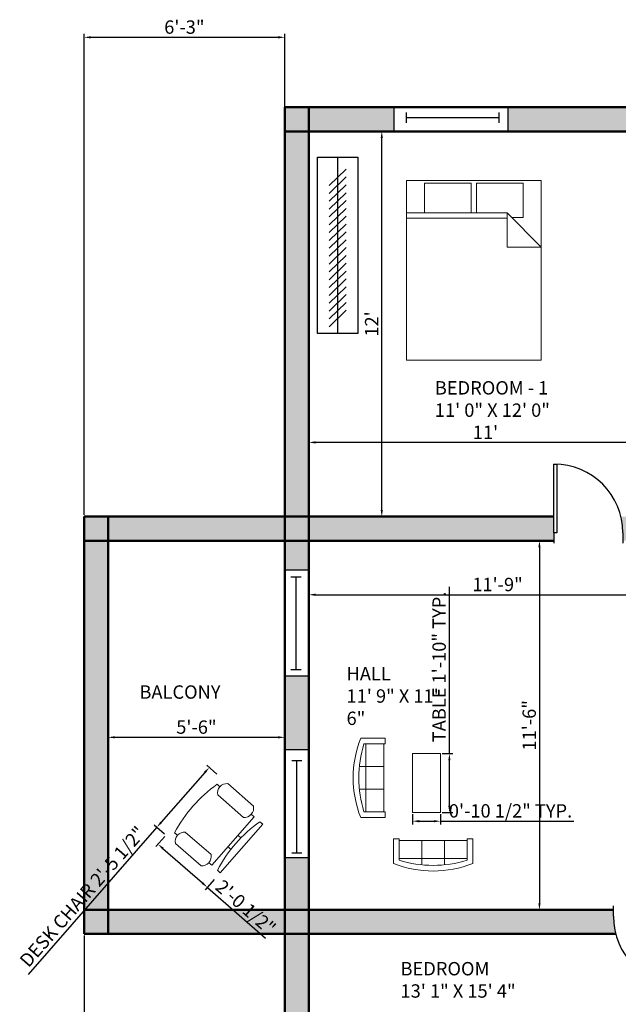
# Model space of a CAD drawing. Units: millimetres. Extents: x 2829 to 4029, y 962 to 1687.
# Tile 2 of 7: x 2829 to 3053, y 1289 to 1657. Entities that reach past the tile are written whole.
import ezdxf

# ---------------------------------------------------------------- set-up
doc = ezdxf.new("R2010")
doc.units = ezdxf.units.MM
for name, color, linetype, lineweight in [('A-ANNO-DIMS', 140, 'Continuous', 18), ('A-AREA-IDEN', 190, 'Continuous', 25), ('A-FLOR-CASE', 90, 'Continuous', 25), ('A-FLOR-CASE-PATT', 90, 'Continuous', 13), ('A-WALL-PATT', 2, 'Continuous', 13), ('doors', 10, 'Continuous', 25), ('furniture', 90, 'Continuous', 18), ('walls', 50, 'Continuous', 50), ('windows', 30, 'Continuous', 25)]:
    doc.layers.add(name, color=color, linetype=linetype, lineweight=lineweight)
doc.styles.get("Standard").update_dxf_attribs({"font": 'arial.ttf'})
doc.dimstyles.new('ISO-25', dxfattribs={"dimtxt": 5, "dimasz": 2.5, "dimexe": 1.25, "dimexo": 0.625, "dimtad": 1, "dimdec": 0, "dimlunit": 3, "dimtxsty": 'Standard', "dimcen": 2.5, "dimadec": 0, "dimazin": 0, "dimtfac": 1, "dimtdec": 0, "dimtmove": 0, "dimatfit": 3, "dimfxl": 1, "dimarcsym": 0})

# ---------------------------------------------------------------- blocks, each defined once
blk = doc.blocks.new('*U2')
for p, q in [((0, 0), (0, -6)), ((40, 0), (40, -6))]:
    blk.add_line(p, q)
blk.add_lwpolyline([(0, 0), (0, 40), (1.75, 40), (1.75, 0)], close=True)
blk.add_arc((0, 0), 40, 0, 90)
blk = doc.blocks.new('*U4')
for p, q in [((0, 4), (0, 0)), ((36, 4), (36, 0)), ((0, 2), (36, 2))]:
    blk.add_line(p, q)
blk = doc.blocks.new('Bed - Queen')
for p, q in [((0, -80.00003), (0, 0)), ((0, 0), (59.99999, 0)), ((59.99999, 0), (59.99999, -80.00003)), ((7.99999, -1.2), (28.79998, -1.2)), ((7.99999, -14.4), (7.99999, -1.2)), ((28.79998, -1.2), (28.79998, -14.4)), ((31.19999, -1.2), (51.99999, -1.2)), ((31.19999, -14.4), (31.19999, -1.2)), ((51.99999, -1.2), (51.99999, -16.4)), ((0, -14.4), (44.8, -14.4)), ((44.8, -16.8), (0, -16.8)), ((59.99999, -29.6), (44.8, -14.4)), ((44.8, -14.4), (44.8, -29.6)), ((51.99999, -16.4), (46.79936, -16.4)), ((44.8, -29.6), (59.99999, -29.6)), ((59.99999, -80.00003), (0, -80.00003))]:
    blk.add_line(p, q)
blk = doc.blocks.new('Sofa - Roundback 7 ft.')
for p, q in [((-12.00002, -32.4421), (-12.00003, -6.5971)), ((11.99997, -32.4421), (11.99998, -6.5971)), ((-36.000027, -34), (-36.000027, -11.4696)), ((-35.999844, -13.3819), (35.9998, -13.3819)), ((35.99998, -34), (35.99998, -11.4696)), ((-36.000027, -32.4421), (35.99998, -32.4421))]:
    blk.add_line(p, q)
for points in [[(-36.000027, -34), (-42.000027, -34), (-42.000027, -8)], [(41.99998, -8), (41.99998, -34), (35.99998, -34)]]:
    blk.add_lwpolyline(points)
for centre, radius, start, end in [((0, -114.25), 114.25, 68.43141, 111.5686), ((-0.00001, -127.1968), 121.1968, 72.72033, 107.2797)]:
    blk.add_arc(centre, radius, start, end)
blk = doc.blocks.new('Chair - Desk')
for p, q in [((-8.5, 0), (-8.5, -1)), ((-8.5, 0), (8.5, 0)), ((8.5, 0), (8.5, -1)), ((-2, -3), (-2, -1.9355)), ((2, -1.9576), (2, -3)), ((-10.5, -5), (-10.5, -14)), ((-8.5, -3), (-8.5, -4)), ((-8.5, -3), (8.5, -3)), ((-6.5, -14), (-6.5, -5)), ((6.5, -5), (6.5, -14)), ((8.5, -3), (8.5, -4)), ((10.5, -14), (10.5, -5)), ((-8.5, -15), (-8.5, -16)), ((8.5, -15), (8.5, -16))]:
    blk.add_line(p, q)
for centre, radius, start, end in [((0, 34.625), 36.625, 256.5803, 283.4197), ((-8.5, -6.5), 2.5, 36.8699, 143.1301), ((8.5, -6.5), 2.5, 36.8699, 143.1301), ((-8.5, -12.5), 2.5, 216.8699, 323.1301), ((8.5, -12.5), 2.5, 216.8699, 323.1301), ((0, 19.625), 36.625, 256.5803, 283.4197)]:
    blk.add_arc(centre, radius, start, end)
blk = doc.blocks.new('*D11')
at = {"layer": 'A-ANNO-DIMS', "color": 0, "lineweight": -2, "transparency": 16777216}
for p, q in [((2969.88, 1615.38), (2963.31, 1615.38)), ((2964.56, 1473.88), (2964.56, 1612.88)), ((2969.88, 1471.38), (2963.31, 1471.38))]:
    blk.add_line(p, q, dxfattribs=at)
at = {"layer": 'A-ANNO-DIMS', "color": 0, "transparency": 16777216}
for points in [[(2964.15, 1612.88), (2964.98, 1612.88), (2964.56, 1615.38)], [(2964.15, 1473.88), (2964.98, 1473.88), (2964.56, 1471.38)]]:
    blk.add_solid(points, dxfattribs=at)
at = {"layer": 'Defpoints', "color": 0, "transparency": 16777216}
for p in [(2964.56, 1615.38), (2970.5, 1615.38), (2970.5, 1471.38)]:
    blk.add_point(p, dxfattribs=at)
at = {"layer": 'A-ANNO-DIMS', "color": 0, "transparency": 16777216, "insert": (2961.43, 1543.38), "char_height": 5, "attachment_point": 5, "rotation": 90}
blk.add_mtext("12'", dxfattribs=at)
blk = doc.blocks.new('*D12')
at = {"layer": 'A-ANNO-DIMS', "color": 0, "lineweight": -2, "transparency": 16777216}
for p, q in [((2937.31, 1499.73), (2937.31, 1500.36)), ((3066.81, 1499.11), (2939.81, 1499.11)), ((3069.31, 1499.73), (3069.31, 1500.36))]:
    blk.add_line(p, q, dxfattribs=at)
at = {"layer": 'A-ANNO-DIMS', "color": 0, "transparency": 16777216}
for points in [[(2939.81, 1499.52), (2939.81, 1498.69), (2937.31, 1499.11)], [(3066.81, 1499.52), (3066.81, 1498.69), (3069.31, 1499.11)]]:
    blk.add_solid(points, dxfattribs=at)
at = {"layer": 'Defpoints', "color": 0, "transparency": 16777216}
for p in [(2937.31, 1499.11), (2937.31, 1499.11), (3069.31, 1499.11)]:
    blk.add_point(p, dxfattribs=at)
at = {"layer": 'A-ANNO-DIMS', "color": 0, "transparency": 16777216, "insert": (3003.31, 1502.24), "char_height": 5, "attachment_point": 5}
blk.add_mtext("11'", dxfattribs=at)
blk = doc.blocks.new('*D19')
at = {"layer": 'A-ANNO-DIMS', "color": 0, "lineweight": -2, "transparency": 16777216}
for p, q in [((2862.31, 1391.61), (2862.31, 1387.63)), ((2928.31, 1391.61), (2928.31, 1387.63)), ((2925.81, 1388.88), (2864.81, 1388.88))]:
    blk.add_line(p, q, dxfattribs=at)
at = {"layer": 'A-ANNO-DIMS', "color": 0, "transparency": 16777216}
for points in [[(2864.81, 1389.3), (2864.81, 1388.47), (2862.31, 1388.88)], [(2925.81, 1389.3), (2925.81, 1388.47), (2928.31, 1388.88)]]:
    blk.add_solid(points, dxfattribs=at)
at = {"layer": 'Defpoints', "color": 0, "transparency": 16777216}
for p in [(2862.31, 1392.23), (2928.31, 1392.23), (2862.31, 1388.88)]:
    blk.add_point(p, dxfattribs=at)
at = {"layer": 'A-ANNO-DIMS', "color": 0, "transparency": 16777216, "insert": (2895.31, 1392.06), "char_height": 5, "attachment_point": 5}
blk.add_mtext('5\'-6"', dxfattribs=at)
blk = doc.blocks.new('*D26')
at = {"layer": 'A-ANNO-DIMS', "color": 0, "lineweight": -2, "transparency": 16777216}
for p, q in [((3020.27, 1462.38), (3024.72, 1462.38)), ((3023.47, 1459.88), (3023.47, 1326.88)), ((3020.27, 1324.38), (3024.72, 1324.38))]:
    blk.add_line(p, q, dxfattribs=at)
at = {"layer": 'A-ANNO-DIMS', "color": 0, "transparency": 16777216}
for points in [[(3023.05, 1459.88), (3023.89, 1459.88), (3023.47, 1462.38)], [(3023.05, 1326.88), (3023.89, 1326.88), (3023.47, 1324.38)]]:
    blk.add_solid(points, dxfattribs=at)
at = {"layer": 'Defpoints', "color": 0, "transparency": 16777216}
for p in [(3019.64, 1462.38), (3019.64, 1324.38), (3023.47, 1324.38)]:
    blk.add_point(p, dxfattribs=at)
at = {"layer": 'A-ANNO-DIMS', "color": 0, "transparency": 16777216, "insert": (3020.29, 1393.38), "char_height": 5, "attachment_point": 5, "rotation": 90}
blk.add_mtext('11\'-6"', dxfattribs=at)
blk = doc.blocks.new('*D27')
at = {"layer": 'A-ANNO-DIMS', "color": 0, "lineweight": -2, "transparency": 16777216}
for p, q in [((2937.31, 1461.76), (2937.31, 1440.93)), ((3078.31, 1461.76), (3078.31, 1440.93)), ((2939.81, 1442.18), (3075.81, 1442.18))]:
    blk.add_line(p, q, dxfattribs=at)
at = {"layer": 'A-ANNO-DIMS', "color": 0, "transparency": 16777216}
for points in [[(2939.81, 1442.59), (2939.81, 1441.76), (2937.31, 1442.18)], [(3075.81, 1442.59), (3075.81, 1441.76), (3078.31, 1442.18)]]:
    blk.add_solid(points, dxfattribs=at)
at = {"layer": 'Defpoints', "color": 0, "transparency": 16777216}
for p in [(2937.31, 1462.38), (3078.31, 1462.38), (3078.31, 1442.18)]:
    blk.add_point(p, dxfattribs=at)
at = {"layer": 'A-ANNO-DIMS', "color": 0, "transparency": 16777216, "insert": (3007.81, 1445.36), "char_height": 5, "attachment_point": 5}
blk.add_mtext('11\'-9"', dxfattribs=at)
blk = doc.blocks.new('TABLE-COFFEE-RECT')
blk.add_lwpolyline([(0, 0), (10.49, 0), (10.49, 21.96), (0, 21.96)], close=True)
blk = doc.blocks.new('*D81')
at = {"layer": 'A-ANNO-DIMS', "color": 0, "lineweight": -2, "transparency": 16777216}
for p, q in [((2902.99, 1375.11), (2899.17, 1378.46)), ((2898.46, 1375.76), (2882.17, 1357.14)), ((2880.52, 1355.26), (2832.4, 1300.26)), ((2883.41, 1352.73), (2879.58, 1356.08))]:
    blk.add_line(p, q, dxfattribs=at)
at = {"layer": 'A-ANNO-DIMS', "color": 0, "transparency": 16777216}
for points in [[(2898.15, 1376.03), (2898.77, 1375.48), (2900.11, 1377.64)], [(2881.85, 1357.41), (2882.48, 1356.86), (2880.52, 1355.26)]]:
    blk.add_solid(points, dxfattribs=at)
at = {"layer": 'Defpoints', "color": 0, "transparency": 16777216}
for p in [(2903.46, 1374.7), (2880.52, 1355.26), (2883.88, 1352.32)]:
    blk.add_point(p, dxfattribs=at)
at = {"layer": 'A-ANNO-DIMS', "color": 0, "transparency": 16777216, "insert": (2853.22, 1328.93), "char_height": 5, "attachment_point": 5, "rotation": 48.8141}
blk.add_mtext('DESK CHAIR 2\'-5 1/2"', dxfattribs=at)
blk = doc.blocks.new('*D82')
at = {"layer": 'A-ANNO-DIMS', "color": 0, "lineweight": -2, "transparency": 16777216}
for p, q in [((2883.47, 1351.85), (2880.12, 1348.02)), ((2882.82, 1347.31), (2897.53, 1334.44)), ((2901.94, 1335.68), (2898.59, 1331.85)), ((2899.42, 1332.79), (2921.07, 1313.84))]:
    blk.add_line(p, q, dxfattribs=at)
at = {"layer": 'A-ANNO-DIMS', "color": 0, "transparency": 16777216}
for points in [[(2883.1, 1347.63), (2882.55, 1347), (2880.94, 1348.96)], [(2897.81, 1334.75), (2897.26, 1334.13), (2899.42, 1332.79)]]:
    blk.add_solid(points, dxfattribs=at)
at = {"layer": 'Defpoints', "color": 0, "transparency": 16777216}
for p in [(2883.88, 1352.32), (2902.35, 1336.15), (2899.42, 1332.79)]:
    blk.add_point(p, dxfattribs=at)
at = {"layer": 'A-ANNO-DIMS', "color": 0, "transparency": 16777216, "insert": (2913.3, 1324.91), "char_height": 5, "attachment_point": 5, "rotation": 318.8141}
blk.add_mtext('2\'-0 1/2"', dxfattribs=at)
blk = doc.blocks.new('*D87')
at = {"layer": 'A-ANNO-DIMS', "color": 0, "lineweight": -2, "transparency": 16777216}
for p, q in [((2989.82, 1382.78), (2989.82, 1445.09)), ((2987.15, 1382.78), (2991.07, 1382.78)), ((2989.82, 1363.33), (2989.82, 1380.28)), ((2987.15, 1360.83), (2991.07, 1360.83))]:
    blk.add_line(p, q, dxfattribs=at)
at = {"layer": 'A-ANNO-DIMS', "color": 0, "transparency": 16777216}
for points in [[(2989.41, 1380.28), (2990.24, 1380.28), (2989.82, 1382.78)], [(2989.41, 1363.33), (2990.24, 1363.33), (2989.82, 1360.83)]]:
    blk.add_solid(points, dxfattribs=at)
at = {"layer": 'Defpoints', "color": 0, "transparency": 16777216}
for p in [(2986.53, 1382.78), (2989.82, 1382.78), (2986.53, 1360.83)]:
    blk.add_point(p, dxfattribs=at)
at = {"layer": 'A-ANNO-DIMS', "color": 0, "transparency": 16777216, "insert": (2986.64, 1415.19), "char_height": 5, "attachment_point": 5, "rotation": 90}
blk.add_mtext('TABLE 1\'-10" TYP.', dxfattribs=at)
blk = doc.blocks.new('*D88')
at = {"layer": 'A-ANNO-DIMS', "color": 0, "lineweight": -2, "transparency": 16777216}
for p, q in [((2976.04, 1360.2), (2976.04, 1356.29)), ((2986.53, 1360.2), (2986.53, 1356.29)), ((2978.54, 1357.54), (2984.03, 1357.54)), ((2986.53, 1357.54), (3036.29, 1357.54))]:
    blk.add_line(p, q, dxfattribs=at)
at = {"layer": 'A-ANNO-DIMS', "color": 0, "transparency": 16777216}
for points in [[(2978.54, 1357.95), (2978.54, 1357.12), (2976.04, 1357.54)], [(2984.03, 1357.95), (2984.03, 1357.12), (2986.53, 1357.54)]]:
    blk.add_solid(points, dxfattribs=at)
at = {"layer": 'Defpoints', "color": 0, "transparency": 16777216}
for p in [(2976.04, 1360.83), (2986.53, 1360.83), (2986.53, 1357.54)]:
    blk.add_point(p, dxfattribs=at)
at = {"layer": 'A-ANNO-DIMS', "color": 0, "transparency": 16777216, "insert": (3012.66, 1360.75), "char_height": 5, "attachment_point": 5}
blk.add_mtext('0\'-10 1/2" TYP.', dxfattribs=at)
blk = doc.blocks.new('*D89')
at = {"layer": 'A-ANNO-DIMS', "color": 0, "lineweight": -2, "transparency": 16777216}
for p, q in [((2853.31, 1314.76), (2853.31, 1094.98)), ((3369.31, 1121.76), (3369.31, 1094.98)), ((2855.81, 1096.23), (3366.81, 1096.23))]:
    blk.add_line(p, q, dxfattribs=at)
at = {"layer": 'A-ANNO-DIMS', "color": 0, "transparency": 16777216}
for points in [[(2855.81, 1096.65), (2855.81, 1095.81), (2853.31, 1096.23)], [(3366.81, 1096.65), (3366.81, 1095.81), (3369.31, 1096.23)]]:
    blk.add_solid(points, dxfattribs=at)
at = {"layer": 'Defpoints', "color": 0, "transparency": 16777216}
for p in [(2853.31, 1315.38), (3369.31, 1122.38), (3369.31, 1096.23)]:
    blk.add_point(p, dxfattribs=at)
at = {"layer": 'A-ANNO-DIMS', "color": 0, "transparency": 16777216, "insert": (3111.31, 1099.41), "char_height": 5, "attachment_point": 5}
blk.add_mtext('43\'-0"', dxfattribs=at)
blk = doc.blocks.new('*D91')
at = {"layer": 'A-ANNO-DIMS', "color": 0, "lineweight": -2, "transparency": 16777216}
for p, q in [((2853.31, 1472.01), (2853.31, 1651.78)), ((2855.81, 1650.53), (2925.81, 1650.53)), ((2928.31, 1472.01), (2928.31, 1651.78))]:
    blk.add_line(p, q, dxfattribs=at)
at = {"layer": 'A-ANNO-DIMS', "color": 0, "transparency": 16777216}
for points in [[(2855.81, 1650.95), (2855.81, 1650.11), (2853.31, 1650.53)], [(2925.81, 1650.95), (2925.81, 1650.11), (2928.31, 1650.53)]]:
    blk.add_solid(points, dxfattribs=at)
at = {"layer": 'Defpoints', "color": 0, "transparency": 16777216}
for p in [(2928.31, 1650.53), (2853.31, 1471.38), (2928.31, 1471.38)]:
    blk.add_point(p, dxfattribs=at)
at = {"layer": 'A-ANNO-DIMS', "color": 0, "transparency": 16777216, "insert": (2890.81, 1653.71), "char_height": 5, "attachment_point": 5}
blk.add_mtext('6\'-3"', dxfattribs=at)

msp = doc.modelspace()

# ---------------------------------------------------------------- hatches: boundary and pattern name
at = {"layer": 'A-FLOR-CASE-PATT'}
h = msp.add_hatch(dxfattribs=at)
h.set_pattern_fill('ANSI31', color=256, scale=0.66617, angle=-1.176, style=0)
h.paths.add_polyline_path([(2951.27, 1602.28), (2944.86, 1596.14), (2944.89, 1540.46), (2951.29, 1546.61)])
at = {"layer": 'A-WALL-PATT'}
h = msp.add_hatch(color=256, dxfattribs=at)
h.dxf.hatch_style = 1
h.paths.add_polyline_path([(2969.05, 1624.38), (2937.31, 1624.38), (2937.31, 1615.38), (2969.05, 1615.38)])
h.paths.add_polyline_path([(2937.31, 1624.38), (2928.31, 1624.38), (2928.31, 1615.38), (2937.31, 1615.38)])
h.paths.add_polyline_path([(2937.31, 1615.38), (2928.31, 1615.38), (2928.31, 1471.38), (2937.31, 1471.38)])
h.paths.add_polyline_path([(3069.31, 1624.38), (3011.61, 1624.38), (3011.61, 1615.38), (3069.31, 1615.38)])
h.paths.add_polyline_path([(3078.31, 1624.38), (3069.31, 1624.38), (3069.31, 1615.38), (3078.31, 1615.38)])
h.paths.add_polyline_path([(3078.31, 1615.38), (3069.31, 1615.38), (3069.31, 1581.62), (3069.43, 1581.62), (3078.31, 1581.62)])
h.paths.add_polyline_path([(3078.31, 1566.24, -0.131652), (3069.43, 1563.86), (3069.31, 1563.86), (3069.31, 1519.38), (3078.31, 1519.38)])
h.paths.add_polyline_path([(3078.31, 1519.38), (3069.31, 1519.38), (3069.31, 1510.38), (3078.31, 1510.38)])
h.paths.add_polyline_path([(3138.31, 1519.38), (3078.31, 1519.38), (3078.31, 1510.38), (3138.31, 1510.38)])
h.paths.add_polyline_path([(3147.31, 1519.38), (3138.31, 1519.38), (3138.31, 1510.38), (3147.31, 1510.38)])
h.paths.add_polyline_path([(3147.31, 1615.38), (3138.31, 1615.38), (3138.31, 1519.38), (3147.31, 1519.38)])
h.paths.add_polyline_path([(3147.31, 1624.38), (3138.31, 1624.38), (3138.31, 1615.38), (3147.31, 1615.38)])
h.paths.add_polyline_path([(3138.31, 1624.38), (3116.25, 1624.38), (3116.25, 1615.38), (3138.31, 1615.38)])
h.paths.add_polyline_path([(3096.9, 1624.38), (3078.31, 1624.38), (3078.31, 1615.38), (3096.9, 1615.38)])
h.paths.add_polyline_path([(3167.88, 1624.38), (3147.31, 1624.38), (3147.31, 1615.38), (3167.88, 1615.38)])
h.paths.add_polyline_path([(3207.31, 1624.38), (3186.66, 1624.38), (3186.66, 1615.38), (3207.31, 1615.38)])
h.paths.add_polyline_path([(3216.31, 1624.38), (3207.31, 1624.38), (3207.31, 1615.38), (3216.31, 1615.38)])
h.paths.add_polyline_path([(3216.31, 1615.38), (3207.31, 1615.38), (3207.31, 1585.36), (3216.31, 1585.36)])
h.paths.add_polyline_path([(3216.31, 1567.6), (3216.21, 1567.6, -0.131958), (3207.31, 1569.99), (3207.31, 1519.38), (3216.31, 1519.38)])
h.paths.add_polyline_path([(3216.31, 1519.38), (3207.31, 1519.38), (3207.31, 1510.38), (3216.31, 1510.38)])
h.paths.add_polyline_path([(3207.31, 1519.38), (3147.31, 1519.38), (3147.31, 1510.38), (3207.31, 1510.38)])
h.paths.add_polyline_path([(3269.97, 1624.38), (3216.31, 1624.38), (3216.31, 1615.38), (3269.97, 1615.38)])
h.paths.add_polyline_path([(3360.31, 1624.38), (3310.37, 1624.38), (3310.37, 1615.38), (3360.31, 1615.38)])
h.paths.add_polyline_path([(3369.31, 1624.38), (3360.31, 1624.38), (3360.31, 1615.38), (3369.31, 1615.38)])
h.paths.add_polyline_path([(3369.31, 1615.38), (3360.31, 1615.38), (3360.31, 1471.38), (3369.31, 1471.38)])
h.paths.add_polyline_path([(3360.31, 1471.38), (3216.31, 1471.38), (3216.31, 1462.38), (3360.31, 1462.38)])
h.paths.add_polyline_path([(3216.31, 1471.38), (3207.31, 1471.38), (3207.31, 1462.38), (3216.31, 1462.38)])
h.paths.add_polyline_path([(3216.31, 1479.42, -0.089587), (3207.31, 1477.74), (3207.31, 1471.38), (3216.31, 1471.38)])
h.paths.add_polyline_path([(3216.31, 1510.38), (3207.31, 1510.38), (3207.31, 1503.49), (3216.31, 1503.49)])
h.paths.add_polyline_path([(3369.31, 1471.38), (3360.31, 1471.38), (3360.31, 1462.38), (3369.31, 1462.38)])
h.paths.add_polyline_path([(3360.31, 1324.38), (3163.31, 1324.38), (3163.31, 1315.38), (3360.31, 1315.38)])
h.paths.add_polyline_path([(3369.31, 1324.38), (3360.31, 1324.38), (3360.31, 1315.38), (3369.31, 1315.38)])
h.paths.add_polyline_path([(3028.89, 1471.38), (2937.31, 1471.38), (2937.31, 1462.38), (3028.89, 1462.38), (3028.89, 1465.26)])
h.paths.add_polyline_path([(2937.31, 1471.38), (2928.31, 1471.38), (2928.31, 1462.38), (2937.31, 1462.38)])
h.paths.add_polyline_path([(2928.31, 1471.38), (2862.31, 1471.38), (2862.31, 1462.38), (2928.31, 1462.38)])
h.paths.add_polyline_path([(2862.31, 1462.38), (2853.31, 1462.38), (2853.31, 1324.38), (2862.31, 1324.38)])
h.paths.add_polyline_path([(2862.31, 1471.38), (2853.31, 1471.38), (2853.31, 1462.38), (2862.31, 1462.38)])
h.paths.add_polyline_path([(2928.31, 1324.38), (2862.31, 1324.38), (2862.31, 1315.38), (2928.31, 1315.38)])
h.paths.add_polyline_path([(2862.31, 1324.38), (2853.31, 1324.38), (2853.31, 1315.38), (2862.31, 1315.38)])
h.paths.add_polyline_path([(3051.08, 1322.02), (3051.08, 1324.38), (2937.31, 1324.38), (2937.31, 1315.38), (3051.95, 1315.38, -0.065323)])
h.paths.add_polyline_path([(2937.31, 1324.38), (2928.31, 1324.38), (2928.31, 1315.38), (2937.31, 1315.38)])
h.paths.add_polyline_path([(3103.31, 1315.38), (3094.31, 1315.38), (3094.31, 1248.38), (3103.31, 1248.38)])
h.paths.add_polyline_path([(3103.31, 1324.38), (3094.31, 1324.38), (3094.31, 1315.38), (3103.31, 1315.38)])
h.paths.add_polyline_path([(3094.31, 1324.38), (3076.83, 1324.38), (3076.83, 1322.02), (3076.83, 1315.38), (3094.31, 1315.38)])
h.paths.add_polyline_path([(3078.31, 1510.38), (3069.31, 1510.38), (3069.31, 1471.38), (3078.31, 1471.38)])
h.paths.add_polyline_path([(3078.31, 1471.38), (3069.31, 1471.38), (3069.31, 1462.38), (3078.31, 1462.38)])
h.paths.add_polyline_path([(3069.31, 1471.38), (3053.91, 1471.38, -0.060076), (3054.65, 1465.26), (3054.65, 1462.38), (3069.31, 1462.38)])
h.paths.add_polyline_path([(2937.31, 1315.38), (2928.31, 1315.38), (2928.31, 1131.38), (2937.31, 1131.38)])
h.paths.add_polyline_path([(2937.31, 1131.38), (2928.31, 1131.38), (2928.31, 1122.38), (2937.31, 1122.38)])
h.paths.add_polyline_path([(2978.9, 1131.38), (2937.31, 1131.38), (2937.31, 1122.38), (2978.9, 1122.38)])
h.paths.add_polyline_path([(3094.31, 1131.38), (3017.24, 1131.38), (3017.24, 1122.38), (3094.31, 1122.38)])
h.paths.add_polyline_path([(3103.31, 1131.38), (3094.31, 1131.38), (3094.31, 1122.38), (3103.31, 1122.38)])
h.paths.add_polyline_path([(3103.31, 1179.58, -0.112378), (3095.63, 1177.83), (3094.31, 1177.83), (3094.31, 1131.38), (3103.31, 1131.38)])
h.paths.add_polyline_path([(3103.31, 1239.38), (3094.31, 1239.38), (3094.31, 1195.59), (3095.63, 1195.59), (3103.31, 1195.59)])
h.paths.add_polyline_path([(3103.31, 1248.38), (3094.31, 1248.38), (3094.31, 1239.38), (3103.31, 1239.38)])
h.paths.add_polyline_path([(3163.31, 1248.38), (3103.31, 1248.38), (3103.31, 1239.38), (3163.31, 1239.38)])
h.paths.add_polyline_path([(3172.31, 1248.38), (3163.31, 1248.38), (3163.31, 1239.38), (3172.31, 1239.38)])
h.paths.add_polyline_path([(3172.31, 1239.38), (3163.31, 1239.38), (3163.31, 1197.38), (3172.31, 1197.38)])
h.paths.add_polyline_path([(3172.31, 1197.38), (3163.31, 1197.38), (3163.31, 1188.38), (3172.31, 1188.38)])
h.paths.add_polyline_path([(3172.31, 1188.38), (3163.31, 1188.38), (3163.31, 1131.38), (3172.31, 1131.38)])
h.paths.add_polyline_path([(3172.31, 1131.38), (3163.31, 1131.38), (3163.31, 1122.38), (3172.31, 1122.38)])
h.paths.add_polyline_path([(3163.31, 1131.38), (3143.05, 1131.38), (3143.05, 1122.38), (3163.31, 1122.38)])
h.paths.add_polyline_path([(3123.82, 1131.38), (3103.31, 1131.38), (3103.31, 1122.38), (3123.82, 1122.38)])
h.paths.add_polyline_path([(3273.8, 1131.38), (3172.31, 1131.38), (3172.31, 1122.38), (3273.8, 1122.38)])
h.paths.add_polyline_path([(3360.31, 1131.38), (3293.49, 1131.38), (3293.49, 1122.38), (3360.31, 1122.38)])
h.paths.add_polyline_path([(3369.31, 1131.38), (3360.31, 1131.38), (3360.31, 1122.38), (3369.31, 1122.38)])
h.paths.add_polyline_path([(3369.31, 1188.38), (3360.31, 1188.38), (3360.31, 1131.38), (3369.31, 1131.38)])
h.paths.add_polyline_path([(3369.31, 1197.38), (3360.31, 1197.38), (3360.31, 1188.38), (3369.31, 1188.38)])
h.paths.add_polyline_path([(3360.31, 1197.38), (3252.19, 1197.38), (3252.19, 1188.38), (3360.31, 1188.38)])
h.paths.add_polyline_path([(3234.43, 1197.38), (3172.31, 1197.38), (3172.31, 1188.38), (3237.05, 1188.38, -0.134312)])
h.paths.add_polyline_path([(3369.31, 1315.38), (3360.31, 1315.38), (3360.31, 1197.38), (3369.31, 1197.38)])
edge = h.paths.add_edge_path()
edge.add_arc((3367.95, 1432.65), 25.75, 90, 107.2357)
edge.add_line((3360.31, 1457.25), (3360.31, 1462.38))
edge.add_line((3360.31, 1462.38), (3369.31, 1462.38))
edge.add_line((3369.31, 1462.38), (3369.31, 1458.41))
edge.add_line((3369.31, 1458.41), (3367.95, 1458.41))
h.paths.add_polyline_path([(3369.31, 1432.65), (3360.31, 1432.65), (3360.31, 1324.38), (3369.31, 1324.38)])
h = msp.add_hatch(color=256, dxfattribs=at)
h.dxf.hatch_style = 1
h.paths.add_polyline_path([(2937.31, 1411.79), (2928.31, 1411.79), (2928.31, 1384.16), (2937.31, 1384.16)])
h.paths.add_polyline_path([(2937.31, 1462.38), (2928.31, 1462.38), (2928.31, 1451.4), (2937.31, 1451.4)])
h.paths.add_polyline_path([(2937.31, 1343.95), (2928.31, 1343.95), (2928.31, 1324.38), (2937.31, 1324.38)])

# ---------------------------------------------------------------- linework, layer by layer
at = {"layer": 'A-FLOR-CASE'}
msp.add_line((2948.09, 1539.82), (2948.09, 1605.79), dxfattribs=at)
msp.add_lwpolyline([(2940.58, 1605.79), (2955.59, 1605.79), (2955.59, 1539.82), (2940.58, 1539.82)], close=True, dxfattribs=at)
at = {"layer": 'walls'}
for p, q in [((2928.31, 1624.38), (2928.31, 1122.38)), ((2928.31, 1624.38), (3369.31, 1624.38)), ((2937.31, 1624.38), (2937.31, 1122.38)), ((2928.31, 1615.38), (3369.31, 1615.38)), ((2853.31, 1471.38), (3028.89, 1471.38)), ((2853.31, 1471.38), (2853.31, 1315.38)), ((2862.31, 1471.38), (2862.31, 1315.38)), ((2928.31, 1471.38), (3028.89, 1471.38)), ((2853.31, 1462.38), (3028.89, 1462.38)), ((2928.31, 1462.38), (3028.89, 1462.38)), ((2853.31, 1324.38), (2937.31, 1324.38)), ((2853.31, 1324.38), (3051.08, 1324.38)), ((2853.31, 1315.38), (2937.31, 1315.38)), ((2853.31, 1315.38), (3051.95, 1315.38))]:
    msp.add_line(p, q, dxfattribs=at)
at = {"layer": 'windows'}
for p, q in [((2969.05, 1624.38), (2969.05, 1615.38)), ((3011.61, 1624.38), (3011.61, 1615.38)), ((2937.31, 1451.4), (2928.31, 1451.4)), ((2937.31, 1411.79), (2928.31, 1411.79)), ((2937.31, 1384.16), (2928.31, 1384.16)), ((2928.31, 1343.95), (2937.31, 1343.95))]:
    msp.add_line(p, q, dxfattribs=at)

# ---------------------------------------------------------------- block references
at = {"layer": 'doors', "xscale": 0.6438655246665308, "yscale": 0.6438655246665308, "zscale": 0.6438655246665308}
msp.add_blockref('*U2', (3028.89, 1465.26), dxfattribs=at)
at = {"layer": 'doors', "xscale": 0.6438655246665308, "yscale": 0.6438655246665308, "zscale": 0.6438655246665308, "rotation": 180}
msp.add_blockref('*U2', (3076.83, 1322.02), dxfattribs=at)
at = {"layer": 'furniture', "xscale": 0.8398385143789401, "yscale": 0.8398385143789401, "zscale": 0.8398385143789401}
msp.add_blockref('Bed - Queen', (2973.75, 1596.99), dxfattribs=at)
at = {"layer": 'furniture'}
for name, p, xscale, yscale, zscale, rotation in [('Sofa - Roundback 7 ft.', (2953.87, 1373.72), 0.3523046889690534, 0.3523046889690534, 0.3523046889690534, 89.99997783100578), ('Chair - Desk', (2912.15, 1347.34), 1.416347355929797, 1.416347355929797, 1.416347355929797, 228.8140748342901), ('Sofa - Roundback 7 ft.', (2983.73, 1338.91), 0.3523046889690534, 0.3523046889690534, 0.3523046889690534, 180)]:
    msp.add_blockref(name, p, dxfattribs=dict(at, xscale=xscale, yscale=yscale, zscale=zscale, rotation=rotation))
msp.add_blockref('TABLE-COFFEE-RECT', (2976.04, 1360.83), dxfattribs=at)
at = {"layer": 'windows', "xscale": 0.9597059461553321, "yscale": 0.9597059461553321, "zscale": 0.9597059461553321}
msp.add_blockref('*U4', (2973.71, 1618.61), dxfattribs=at)
msp.add_blockref('*U4', (2973.71, 1618.61), dxfattribs=at)
at = {"layer": 'windows', "xscale": 0.9597059461553321, "yscale": 0.9597059461553321, "zscale": 0.9597059461553321, "rotation": 90}
for p in [(2934.47, 1414.27), (2934.75, 1345.66)]:
    msp.add_blockref('*U4', p, dxfattribs=at)

# ---------------------------------------------------------------- texts
at = {"layer": 'A-AREA-IDEN', "char_height": 5, "attachment_point": 1}
for s, width, insert in [('BEDROOM - 1 \\P11\' 0" X 12\' 0"', 50.0859, (2984.39, 1522.01)), ('HALL\\P11\' 9" X 11\' 6"', 34.6155, (2951.4, 1415.16)), ('BALCONY', 46.5592, (2874.02, 1408.31)), ('BEDROOM \\P13\' 1" X 15\' 4"', 57.6613, (2971.57, 1304.9))]:
    msp.add_mtext_dynamic_manual_height_columns(s, width=width, gutter_width=12.5, heights=[0], dxfattribs=dict(at, insert=insert))

# ---------------------------------------------------------------- dimensions: what is measured, and where the dimension line sits
at = {"layer": 'A-ANNO-DIMS'}
for base, p1, p2, override, picture, middle in [((2928.31, 1650.53), (2853.31, 1471.38), (2928.31, 1471.38), {"dimdec": 1, "dimlfac": 1, "dimrnd": 0, "dimzin": 1, "dimdsep": 46, "dimlunit": 4, "dimfrac": 2}, '*D91', (2890.81, 1653.71)), ((2937.31, 1499.11), (3069.31, 1499.11), (2937.31, 1499.11), {"dimclrd": 0, "dimclre": 0, "dimclrt": 0}, '*D12', (3003.31, 1502.24)), ((3078.31, 1442.18), (2937.31, 1462.38), (3078.31, 1462.38), {"dimclrd": 0, "dimclre": 0, "dimclrt": 0}, '*D27', (3007.81, 1445.36)), ((2862.31, 1388.88), (2928.31, 1392.23), (2862.31, 1392.23), {"dimclrd": 0, "dimclre": 0, "dimclrt": 0}, '*D19', (2895.31, 1392.06)), ((3369.31, 1096.23), (2853.31, 1315.38), (3369.31, 1122.38), {"dimdec": 1, "dimlfac": 1, "dimrnd": 0, "dimzin": 1, "dimdsep": 46, "dimlunit": 4, "dimfrac": 2}, '*D89', (3111.31, 1099.41))]:
    dim = msp.add_linear_dim(base=base, p1=p1, p2=p2, dimstyle='ISO-25', override=override, dxfattribs=at)
    dim.commit()
    dim.dimension.update_dxf_attribs({"geometry": picture, "text_midpoint": middle})
for base, p1, p2, angle, override, picture, middle in [((2964.56, 1615.38), (2970.5, 1471.38), (2970.5, 1615.38), 90, {"dimclrd": 0, "dimclre": 0, "dimclrt": 0}, '*D11', (2961.43, 1543.38)), ((3023.47, 1324.38), (3019.64, 1462.38), (3019.64, 1324.38), 90, {"dimclrd": 0, "dimclre": 0, "dimclrt": 0}, '*D26', (3020.29, 1393.38)), ((2899.41602, 1332.79327), (2883.87816, 1352.31719), (2902.35393, 1336.15088), 318.81407, {"dimdec": 1, "dimlfac": 1, "dimrnd": 0, "dimzin": 1, "dimdsep": 46, "dimlunit": 4, "dimfrac": 2}, '*D82', (2913.29927, 1324.91112))]:
    dim = msp.add_linear_dim(base=base, p1=p1, p2=p2, angle=angle, dimstyle='ISO-25', override=override, dxfattribs=at)
    dim.commit()
    dim.dimension.update_dxf_attribs({"geometry": picture, "text_midpoint": middle})
for base, p1, p2, angle, text, picture, middle in [((2989.8222, 1382.7842), (2986.5289, 1360.8288), (2986.5289, 1382.7842), 90, 'TABLE <> TYP.', '*D87', (2986.6443, 1415.1878)), ((2880.52, 1355.26), (2903.46, 1374.7), (2883.88, 1352.32), 228.8141, 'DESK CHAIR <>', '*D81', (2853.22, 1328.93))]:
    dim = msp.add_linear_dim(base=base, p1=p1, p2=p2, angle=angle, text=text, dimstyle='ISO-25', override={"dimdec": 1, "dimlfac": 1, "dimrnd": 0, "dimzin": 1, "dimdsep": 46, "dimlunit": 4, "dimfrac": 2}, dxfattribs=at)
    dim.commit()
    dim.dimension.update_dxf_attribs({"geometry": picture, "text_midpoint": middle})
dim = msp.add_linear_dim(base=(2986.53, 1357.54), p1=(2976.04, 1360.83), p2=(2986.53, 1360.83), text='<> TYP.', dimstyle='ISO-25', override={"dimdec": 1, "dimlfac": 1, "dimrnd": 0, "dimzin": 1, "dimdsep": 46, "dimlunit": 4, "dimfrac": 2}, dxfattribs=at)
dim.commit()
dim.dimension.update_dxf_attribs({"geometry": '*D88', "text_midpoint": (3012.66, 1360.75)})

doc.saveas('drawing.dxf')
